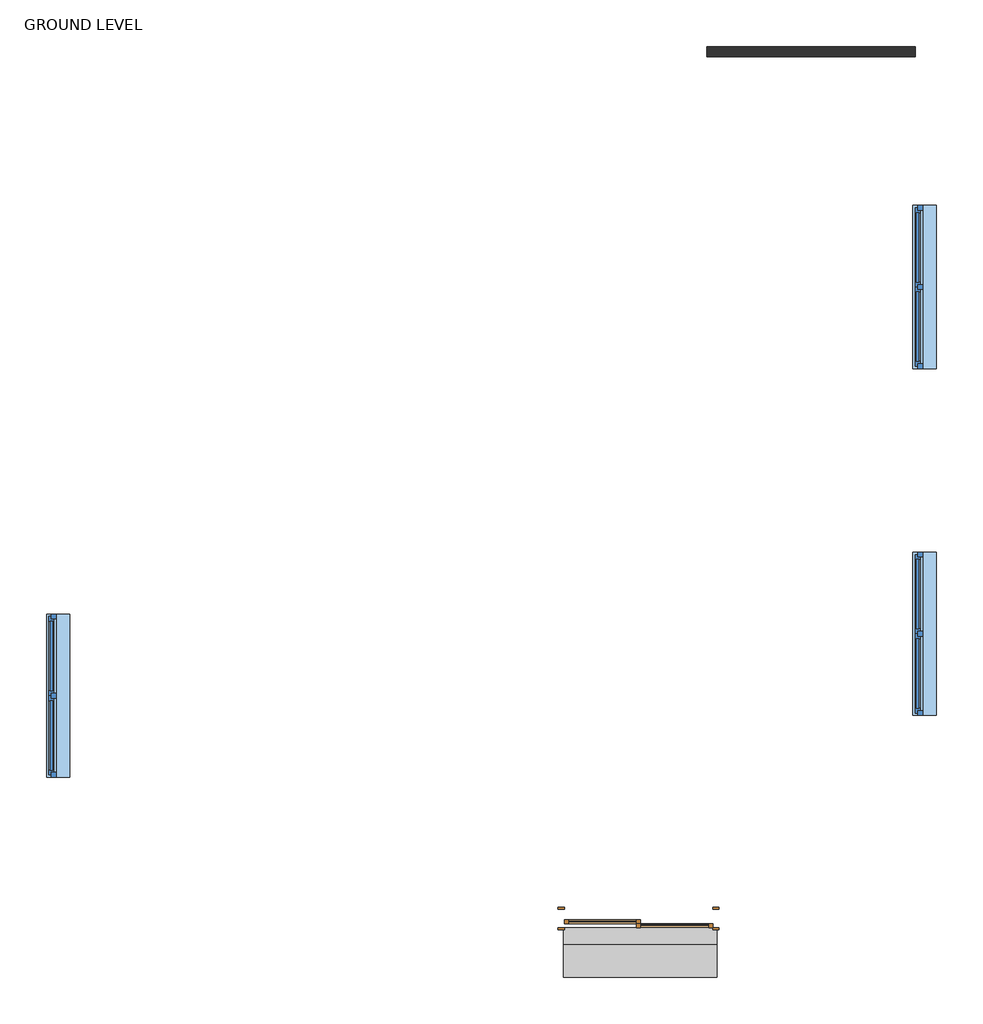
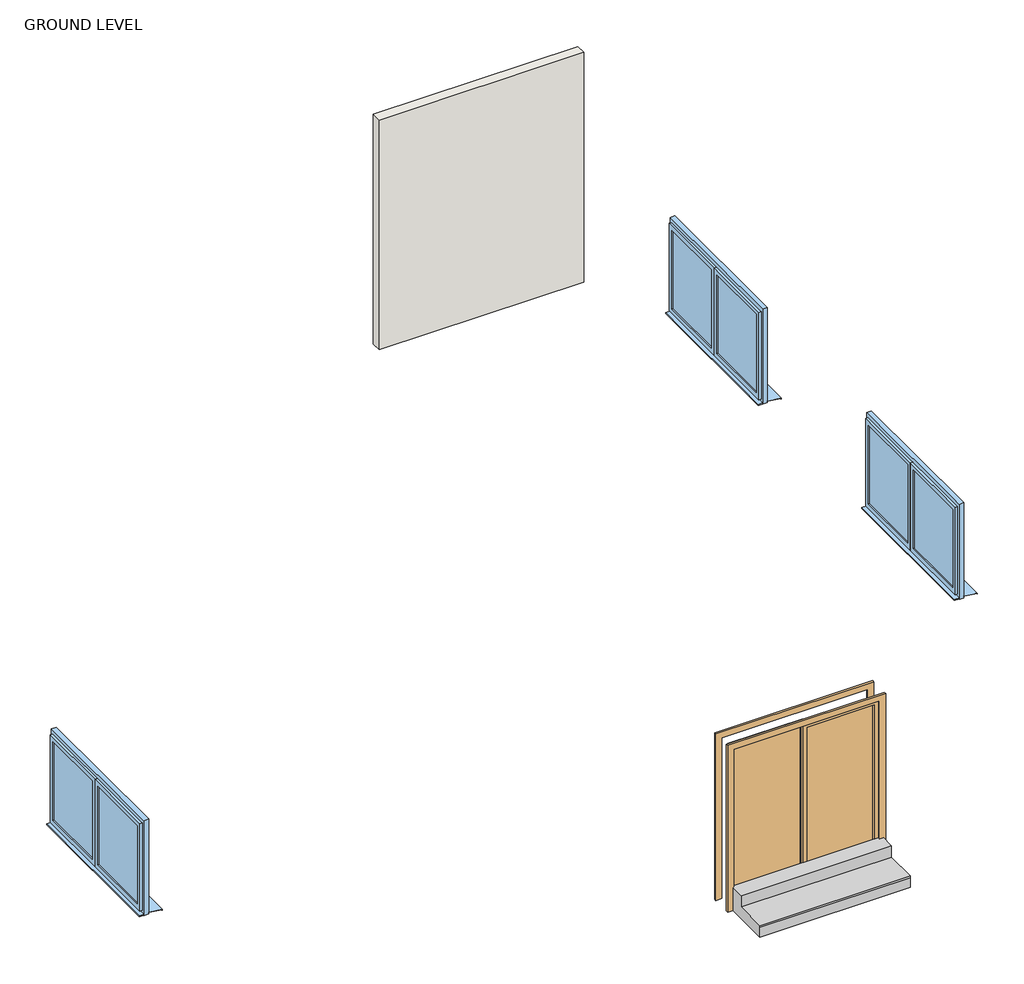
# One storey: 3 windows, 1 door, 1 proxy, 1 wall.
"""IFC4 building model written with IfcOpenShell, lengths in millimetres."""

from ifc_helpers import new_model, si_unit, frame, origin, place, context, project, spatial, polyline, outline, extrude, transform, mapped, element, save
from components import generic_models_9_generic_models_9_d0116728, door_d4d75d1e, w2_w2_7b90d420

model = new_model("IFC4")

# Units and contexts
model_context = context("Model", 3, world=origin())
ifc_project = project(units=[si_unit("LENGTHUNIT", "METRE", prefix="MILLI")], contexts=[model_context])

# Site, building, storey
site = spatial("IfcSite", under=ifc_project)
building = spatial("IfcBuilding", under=site)
storey = spatial("IfcBuildingStorey", under=building, Name="GROUND LEVEL", Elevation=0.0)

# Proxy
placement = place(None, origin())
generic_models_9_generic_models_9_shape = generic_models_9_generic_models_9_d0116728(model_context)
element("IfcBuildingElementProxy", 1, Name="Generic Models 9 : Generic Models 9", ObjectType="Generic Models 9 : Generic Models 9", at=placement, inside=storey, context=model_context, shape_type="MappedRepresentation", body=[
    mapped(generic_models_9_generic_models_9_shape, transform((0.0, 0.0, 0.0), x_axis=(1.0, 0.0, 0.0), y_axis=(0.0, 1.0, 0.0), z_axis=(0.0, 0.0, 1.0))),
])

# Door
door_shape = door_d4d75d1e(model_context)
element("IfcDoor", 2, ObjectType="Door-Double-Sliding : 72\" x 84\"", at=placement, inside=storey, context=model_context, shape_type="MappedRepresentation", body=[
    mapped(door_shape, transform((502.1297209, -4030.9938352, 0.0), x_axis=(-1.0, 0.0, 0.0), y_axis=(0.0, -1.0, 0.0), z_axis=(0.0, 0.0, 1.0))),
])

# Wall
element("IfcWall", 3, ObjectType="INTERIOR WALL 5\"", at=placement, inside=storey, context=model_context, shape_type="SweptSolid", body=[
    extrude(outline(polyline([(3911.3525369, 6446.5061648), (1345.9525369, 6446.5061648), (1345.9525369, 6573.5061648), (3911.3525369, 6573.5061648), (3911.3525369, 6446.5061648)])), frame((0.0, 0.0, 304.8), z_axis=(0.0, 0.0, 1.0), x_axis=(1.0, 0.0, 0.0)), (0.0, 0.0, 1.0), 3048.0),
])

# Windows
w2_w2_shape = w2_w2_7b90d420(model_context)
element("IfcWindow", 4, ObjectType="w2 : w2", at=placement, inside=storey, context=model_context, shape_type="MappedRepresentation", body=[
    mapped(w2_w2_shape, transform((4025.6525369, -652.7938352, 0.0), x_axis=(0.0, -1.0, 0.0), y_axis=(1.0, 0.0, 0.0), z_axis=(0.0, 0.0, 1.0))),
])
element("IfcWindow", 5, ObjectType="w2 : w2", at=placement, inside=storey, context=model_context, shape_type="MappedRepresentation", body=[
    mapped(w2_w2_shape, transform((4025.6525369, 3614.4061648, 0.0), x_axis=(0.0, -1.0, 0.0), y_axis=(1.0, 0.0, 0.0), z_axis=(0.0, 0.0, 1.0))),
])
element("IfcWindow", 6, ObjectType="w2 : w2", at=placement, inside=storey, context=model_context, shape_type="MappedRepresentation", body=[
    mapped(w2_w2_shape, transform((-6642.3474631, -1414.7938352, 0.0), x_axis=(0.0, -1.0, 0.0), y_axis=(1.0, 0.0, 0.0), z_axis=(0.0, 0.0, 1.0))),
])

save(model, "model.ifc")

# Revit data of these elements
# Type "Door-Double-Sliding : 72\" x 84\""
#   Type Mark = "8"
#   Construction Type Id = "opn-d45"
#   Assembly Code = "C1020"
#   Analytic Construction = "Wood frame, double glass door "
#   Thickness = 0' - 2"
#   Thermal Resistance (R) = 1.8150 (h·ft²·°F)/BTU
#   Heat Transfer Coefficient (U) = 0.5510 BTU/(h·ft²·°F)
#   Height = 7' - 0"
#   Rail Width = 0' - 2"
#   Stiles = 0' - 2"
#   Trim Projection Ext = 0' - 1"
#   Trim Projection Int = 0' - 1"
#   Trim Width = 0' - 3"
#   Width = 6' - 0"
#   Define Thermal Properties by = 1
#   Glazing = Glass
#   Panel Material = Wood - Birch - Solid Stained Light Low Gloss
#   Trim Material = Paint - Sienna
#   Visual Light Transmittance = 0
#   Solar Heat Gain Coefficient = 0
#   Function = (empty or 0)
#   Wall Closure = (empty or 0)
# Type "INTERIOR WALL 5\""
#   Assembly Code = "B2010"
#   Layers, outside or top first: 0' - 5" "OFF WHITE COLOUR" (function 1)
# Type "w2 : w2"
#   Type Mark = "18"
#   Operation = "DoublePanelVertical"
#   Keynote = "16.05.01"
#   Analytic Construction = "<None>"
#   Rough Width = 6' - 7.13386"
#   Rough Height = 4' - 1.6063"
#   Rahmentiefe = 0' - 2.3622"
#   Rahmenhöhe unten = 0' - 3.14961"
#   Rahmehöhe oben = 0' - 3.14961"
#   Rahmenbreite = 0' - 2.3622"
#   Heat Transfer Coefficient (U) = 2.81836 BTU/(h·ft²·°F)
#   Height = 4' - 1.6063"
#   Flügeltiefe = 0' - 2.3622"
#   Flügelbreite = 0' - 2.3622"
#   Einbautiefe (von außen) [instance default] = 0' - 5.51181"
#   Width = 6' - 7.13386"
#   Kippflügel [instance default] = yes
#   Drehflügel im Grundriß darstellen [instance default] = no
#   Drehflügel [instance default] = yes
#   Define Thermal Properties by = 1
#   Rahmen [instance default] = none
#   Glas [instance default] = blue glass
#   Flügel [instance default] = WINDOW COLOUR WHITE
#   Fensterbank aussen [instance default] = WINDOW COLOUR WHITE
#   Fensterbank innen [instance default] = WINDOW COLOUR WHITE
#   Visual Light Transmittance = 0
#   Thermal Resistance (R) = 0
#   Solar Heat Gain Coefficient = 0
#   Wall Closure = (empty or 0)
# Element 1 (IfcBuildingElementProxy, "Generic Models 9 : Generic Models 9")
#   Phase Created = New Construction
#   Materials on its faces: "Concrete, Cast-in-Place gray"
# Element 2 (IfcDoor, "Door-Double-Sliding : 72\" x 84\"")
#   Phase Created = New Construction
#   Materials on its faces: "Paint - Sienna", "Wood - Birch - Solid Stained Light Low Gloss", "Glass"
# Element 3 (IfcWall, "INTERIOR WALL 5\"")
#   built-in parameter 1001111 = 1' - 0"
#   Top Offset = 0' - 0"
#   Base Offset = 1' - 0"
#   wall height = 10' - 0"
#   Phase Created = New Construction
#   Base Constraint = GROUND LEVEL
#   Top Constraint = FIRST FLR
#   Materials on its faces: "OFF WHITE COLOUR"
# Element 4 (IfcWindow, "w2 : w2")
#   Mark = "1"
#   Einbautiefe (von außen) = 0' - 5.51181"
#   Kippflügel = yes
#   Drehflügel im Grundriß darstellen = no
#   Drehflügel = yes
#   Rahmen = none
#   Glas = blue glass
#   Flügel = WINDOW COLOUR WHITE
#   Fensterbank innen = WINDOW COLOUR WHITE
#   Fensterbank aussen = WINDOW COLOUR WHITE
#   Phase Created = New Construction
#   Materials on its faces: "WINDOW COLOUR WHITE", "blue glass"
# Element 5 (IfcWindow, "w2 : w2")
#   Mark = "2"
#   Einbautiefe (von außen) = 0' - 5.51181"
#   Kippflügel = yes
#   Drehflügel im Grundriß darstellen = no
#   Drehflügel = yes
#   Rahmen = none
#   Glas = blue glass
#   Flügel = WINDOW COLOUR WHITE
#   Fensterbank innen = WINDOW COLOUR WHITE
#   Fensterbank aussen = WINDOW COLOUR WHITE
#   Phase Created = New Construction
#   Materials on its faces: "WINDOW COLOUR WHITE", "blue glass"
# Element 6 (IfcWindow, "w2 : w2")
#   Mark = "3"
#   Einbautiefe (von außen) = 0' - 5.51181"
#   Kippflügel = yes
#   Drehflügel im Grundriß darstellen = no
#   Drehflügel = yes
#   Rahmen = none
#   Glas = blue glass
#   Flügel = WINDOW COLOUR WHITE
#   Fensterbank innen = WINDOW COLOUR WHITE
#   Fensterbank aussen = WINDOW COLOUR WHITE
#   Phase Created = New Construction
#   Materials on its faces: "WINDOW COLOUR WHITE", "blue glass"
# Materials
#   "Glass": class "Glass", colour RGB 0 128 192, transparency 0.75, Description = "Soda Lime Glass", Cost = 0
#   "Wood - Birch - Solid Stained Light Low Gloss": class "Wood", colour RGB 210 159 95, transparency 0, Cost = 0
#   "Paint - Sienna": colour RGB 118 70 51, transparency 0, Cost = 0
#   "OFF WHITE COLOUR": class "Generic", colour RGB 120 120 120, transparency 0, Cost = 0
#   "blue glass": class "System", colour RGB 0 0 255, transparency 0.75, Cost = 0
#   "WINDOW COLOUR WHITE": class "Generic", colour RGB 120 120 120, transparency 0, Cost = 0
#   "Concrete, Cast-in-Place gray": class "Concrete", colour RGB 192 192 192, transparency 0, Description = "Cast-in-place concrete", Cost = 0
